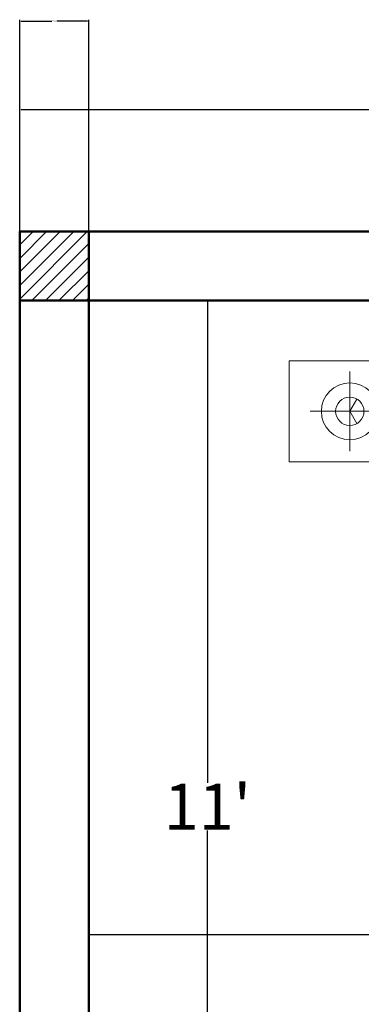
# Model space of a CAD drawing. Units: inches. Extents: x 0 to 281, y -535 to 46.
# Tile 14 of 22: x 27 to 72, y -82 to 46. Entities that reach past the tile are written whole.
import ezdxf

# ---------------------------------------------------------------- set-up
doc = ezdxf.new("R2010")
doc.units = ezdxf.units.IN
doc.header["$MEASUREMENT"] = 0
for name, color, linetype, lineweight in [('A-ANNO-DIMS', 2, 'Continuous', 18), ('A-COLS-PATT', 152, 'Continuous', 13), ('A-FURN', 8, 'Continuous', 18), ('A-WALL', 7, 'Continuous', 50)]:
    doc.layers.add(name, color=color, linetype=linetype, lineweight=lineweight)
doc.styles.get("Standard").update_dxf_attribs({"font": 'arial.ttf'})
doc.dimstyles.get("Standard").update_dxf_attribs({"dimtxt": 0.18, "dimasz": 0.18, "dimexe": 0.18, "dimexo": 0.0625, "dimgap": 0.09, "dimtad": 0, "dimtih": 1, "dimtoh": 1, "dimdec": 0, "dimzin": 0, "dimdsep": 46, "dimlunit": 3, "dimtxsty": 'Standard', "dimcen": 0.09, "dimadec": 0, "dimazin": 0, "dimtfac": 1, "dimtdec": 0, "dimtofl": 0, "dimtmove": 0, "dimatfit": 3, "dimfxl": 1, "dimtolj": 1, "dimtzin": 0, "dimarcsym": 0})

# ---------------------------------------------------------------- blocks, each defined once
blk = doc.blocks.new('*D1')
at = {"layer": 'A-ANNO-DIMS', "color": 0, "lineweight": -2, "transparency": 16777216}
for p, q in [((51.94, 9.41), (51.94, -53.31)), ((52, 9.59), (52.12, 9.59)), ((51.94, -122.23), (51.94, -59.51)), ((52, -122.41), (52.12, -122.41))]:
    blk.add_line(p, q, dxfattribs=at)
at = {"layer": 'A-ANNO-DIMS', "color": 0, "transparency": 16777216}
for points in [[(51.91, 9.41), (51.97, 9.41), (51.94, 9.59)], [(51.91, -122.23), (51.97, -122.23), (51.94, -122.41)]]:
    blk.add_solid(points, dxfattribs=at)
at = {"layer": 'Defpoints', "color": 0, "transparency": 16777216}
for p in [(51.94, 9.59), (51.94, -122.41), (51.94, -122.41)]:
    blk.add_point(p, dxfattribs=at)
at = {"layer": 'A-ANNO-DIMS', "color": 0, "transparency": 16777216, "insert": (51.94, -56.41), "char_height": 6, "attachment_point": 5}
blk.add_mtext("\\A1;11'", dxfattribs=at)
blk = doc.blocks.new('*D2')
at = {"layer": 'A-ANNO-DIMS', "color": 0, "lineweight": -2, "transparency": 16777216}
for p, q in [((36.46, -73.03), (36.46, -72.91)), ((36.64, -73.09), (91.56, -73.09)), ((156.28, -73.09), (101.36, -73.09)), ((156.46, -73.03), (156.46, -72.91))]:
    blk.add_line(p, q, dxfattribs=at)
at = {"layer": 'A-ANNO-DIMS', "color": 0, "transparency": 16777216}
for points in [[(36.64, -73.06), (36.64, -73.12), (36.46, -73.09)], [(156.28, -73.06), (156.28, -73.12), (156.46, -73.09)]]:
    blk.add_solid(points, dxfattribs=at)
at = {"layer": 'Defpoints', "color": 0, "transparency": 16777216}
for p in [(36.46, -73.09), (156.46, -73.09), (156.46, -73.09)]:
    blk.add_point(p, dxfattribs=at)
at = {"layer": 'A-ANNO-DIMS', "color": 0, "transparency": 16777216, "insert": (96.46, -73.09), "char_height": 6, "attachment_point": 5}
blk.add_mtext("\\A1;10'", dxfattribs=at)
blk = doc.blocks.new('*D17')
at = {"layer": 'A-ANNO-DIMS', "color": 0, "lineweight": -2, "transparency": 16777216}
for p, q in [((27.46, 18.65), (27.46, 34.69)), ((243.46, 18.65), (243.46, 34.69)), ((27.64, 34.51), (130.56, 34.51)), ((243.28, 34.51), (140.36, 34.51))]:
    blk.add_line(p, q, dxfattribs=at)
at = {"layer": 'A-ANNO-DIMS', "color": 0, "transparency": 16777216}
for points in [[(27.64, 34.54), (27.64, 34.48), (27.46, 34.51)], [(243.28, 34.54), (243.28, 34.48), (243.46, 34.51)]]:
    blk.add_solid(points, dxfattribs=at)
at = {"layer": 'Defpoints', "color": 0, "transparency": 16777216}
for p in [(243.46, 34.51), (27.46, 18.59), (243.46, 18.59)]:
    blk.add_point(p, dxfattribs=at)
at = {"layer": 'A-ANNO-DIMS', "color": 0, "transparency": 16777216, "insert": (135.46, 34.51), "char_height": 6, "attachment_point": 5}
blk.add_mtext("\\A1;18'", dxfattribs=at)
blk = doc.blocks.new('BEDSIDE-LAMP')
for p, q in [((5.17, 0), (5.17, 10.35)), ((0, 5.17), (10.35, 5.17))]:
    blk.add_line(p, q)
for points in [[(5.17, 5.17), (4.25, 6.77)], [(5.17, 5.17), (4.25, 3.57)]]:
    blk.add_lwpolyline(points)
for radius in [3.7, 1.85]:
    blk.add_circle((5.17, 5.17), radius)
blk = doc.blocks.new('*D40')
at = {"layer": 'A-ANNO-DIMS', "color": 0, "lineweight": -2, "transparency": 16777216}
for p, q in [((27.46, 18.65), (27.46, 46.22)), ((27.64, 46.04), (31.63, 46.04)), ((36.28, 46.04), (32.29, 46.04)), ((36.46, 18.65), (36.46, 46.22))]:
    blk.add_line(p, q, dxfattribs=at)
at = {"layer": 'A-ANNO-DIMS', "color": 0, "transparency": 16777216}
for points in [[(27.64, 46.07), (27.64, 46.01), (27.46, 46.04)], [(36.28, 46.07), (36.28, 46.01), (36.46, 46.04)]]:
    blk.add_solid(points, dxfattribs=at)
at = {"layer": 'Defpoints', "color": 0, "transparency": 16777216}
for p in [(36.46, 46.04), (27.46, 18.59), (36.46, 18.59)]:
    blk.add_point(p, dxfattribs=at)
at = {"layer": 'A-ANNO-DIMS', "color": 0, "transparency": 16777216, "insert": (31.96, 46.04), "char_height": 0.18, "attachment_point": 5}
blk.add_mtext('\\A1;0\'-9"', dxfattribs=at)

msp = doc.modelspace()

# ---------------------------------------------------------------- hatches: boundary and pattern name
at = {"layer": 'A-COLS-PATT'}
h = msp.add_hatch(dxfattribs=at)
h.set_pattern_fill('ANSI31', color=256, scale=10)
h.paths.add_polyline_path([(36.46, 18.59), (27.46, 18.59), (27.46, 9.59), (36.46, 9.59)])
h.paths.add_polyline_path([(165.46, 18.59), (156.46, 18.59), (156.46, 9.59), (165.46, 9.59)])
h.paths.add_polyline_path([(243.46, 18.59), (234.46, 18.59), (234.46, 9.59), (243.46, 9.59)])
h.paths.add_polyline_path([(243.46, -122.41), (234.46, -122.41), (234.46, -131.41), (243.46, -131.41)])
h.paths.add_polyline_path([(36.46, -122.41), (27.46, -122.41), (27.46, -131.41), (36.46, -131.41)])
h.paths.add_polyline_path([(36.46, -498.41), (27.46, -498.41), (27.46, -507.41), (36.46, -507.41)])
h.paths.add_polyline_path([(243.46, -498.41), (234.46, -498.41), (234.46, -507.41), (243.46, -507.41)])
h.paths.add_polyline_path([(159.46, -498.41), (150.46, -498.41), (150.46, -507.41), (159.46, -507.41)])
h.paths.add_polyline_path([(36.46, -392.41), (27.46, -392.41), (27.46, -401.41), (36.46, -401.41)])
h.paths.add_polyline_path([(159.46, -392.41), (150.46, -392.41), (150.46, -401.41), (159.46, -401.41)])
h.paths.add_polyline_path([(243.46, -392.41), (234.46, -392.41), (234.46, -401.41), (243.46, -401.41)])
h.paths.add_polyline_path([(36.46, -263.41), (27.46, -263.41), (27.46, -272.41), (36.46, -272.41)])
h.paths.add_polyline_path([(243.46, -263.41), (234.46, -263.41), (234.46, -272.41), (243.46, -272.41)])

# ---------------------------------------------------------------- linework, layer by layer
at = {"layer": 'A-FURN'}
msp.add_line((62.57, 1.74), (141.76, 1.74), dxfattribs=at)
msp.add_lwpolyline([(78.4, -11.45), (62.57, -11.45), (62.57, 1.74)], dxfattribs=at)
at = {"layer": 'A-WALL'}
for p, q in [((27.46, 18.59), (27.46, -507.41)), ((27.46, 18.59), (243.46, 18.59)), ((36.46, 18.59), (36.46, -507.41)), ((27.46, 9.59), (243.46, 9.59))]:
    msp.add_line(p, q, dxfattribs=at)

# ---------------------------------------------------------------- block references
at = {"layer": 'A-FURN', "rotation": 180}
msp.add_blockref('BEDSIDE-LAMP', (75.66, 0.32), dxfattribs=at)

# ---------------------------------------------------------------- dimensions: what is measured, and where the dimension line sits
at = {"layer": 'A-ANNO-DIMS'}
for base, p1, p2, override, picture, middle in [((36.46, 46.04), (27.46, 18.59), (36.46, 18.59), {"dimdec": 1, "dimlfac": 1, "dimrnd": 0, "dimzin": 1, "dimdsep": 46, "dimlunit": 4, "dimfrac": 2}, '*D40', (31.96, 46.04)), ((243.46, 34.51), (27.46, 18.59), (243.46, 18.59), {"dimtxt": 6, "dimclrd": 0, "dimclre": 0, "dimclrt": 0}, '*D17', (135.46, 34.51)), ((156.46, -73.09), (36.46, -73.09), (156.46, -73.09), {"dimtxt": 6, "dimclrd": 0, "dimclre": 0, "dimclrt": 0}, '*D2', (96.46, -73.09))]:
    dim = msp.add_linear_dim(base=base, p1=p1, p2=p2, dimstyle='Standard', override=override, dxfattribs=at)
    dim.commit()
    dim.dimension.update_dxf_attribs({"geometry": picture, "text_midpoint": middle})
dim = msp.add_linear_dim(base=(51.94, -122.41), p1=(51.94, 9.59), p2=(51.94, -122.41), angle=90, dimstyle='Standard', override={"dimtxt": 6, "dimclrd": 0, "dimclre": 0, "dimclrt": 0}, dxfattribs=at)
dim.commit()
dim.dimension.update_dxf_attribs({"geometry": '*D1', "text_midpoint": (51.94, -56.41)})

doc.saveas('drawing.dxf')
